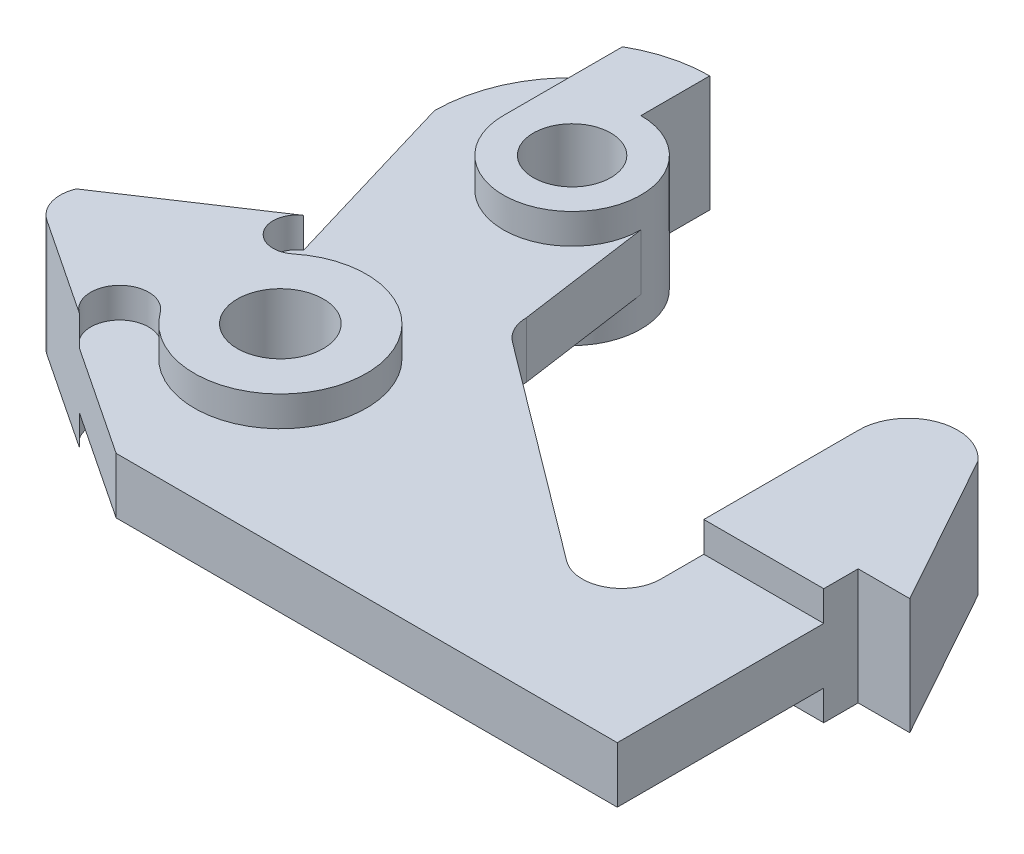
ISO-10303-21;
HEADER;
FILE_DESCRIPTION(('STEP AP214'),'2;1');
FILE_NAME('part.step','',(''),(''),'','','');
FILE_SCHEMA(('AUTOMOTIVE_DESIGN { 1 0 10303 214 1 1 1 1 }'));
ENDSEC;
DATA;
#1=APPLICATION_CONTEXT('core data for automotive mechanical design processes');
#2=APPLICATION_PROTOCOL_DEFINITION('international standard','automotive_design',2000,#1);
#3=PRODUCT_CONTEXT('',#1,'mechanical');
#4=PRODUCT('Part','Part','',(#3));
#5=PRODUCT_RELATED_PRODUCT_CATEGORY('part','',(#4));
#6=PRODUCT_DEFINITION_FORMATION('','',#4);
#7=PRODUCT_DEFINITION_CONTEXT('part definition',#1,'design');
#8=PRODUCT_DEFINITION('design','',#6,#7);
#9=PRODUCT_DEFINITION_SHAPE('','',#8);
#10=(LENGTH_UNIT() NAMED_UNIT(*) SI_UNIT(.MILLI.,.METRE.));
#11=(NAMED_UNIT(*) PLANE_ANGLE_UNIT() SI_UNIT($,.RADIAN.));
#12=(NAMED_UNIT(*) SI_UNIT($,.STERADIAN.) SOLID_ANGLE_UNIT());
#13=UNCERTAINTY_MEASURE_WITH_UNIT(LENGTH_MEASURE(1.E-05),#10,'distance_accuracy_value','');
#14=(GEOMETRIC_REPRESENTATION_CONTEXT(3) GLOBAL_UNCERTAINTY_ASSIGNED_CONTEXT((#13)) GLOBAL_UNIT_ASSIGNED_CONTEXT((#10,
#11,#12)) REPRESENTATION_CONTEXT('',''));
#15=CARTESIAN_POINT('',(0.,0.,0.));
#16=DIRECTION('',(0.,0.,1.));
#17=DIRECTION('',(1.,0.,0.));
#18=AXIS2_PLACEMENT_3D('',#15,#16,#17);
#19=CARTESIAN_POINT('',(0.,13.,0.));
#20=DIRECTION('',(0.,1.,0.));
#21=DIRECTION('',(0.,0.,1.));
#22=AXIS2_PLACEMENT_3D('',#19,#20,#21);
#23=PLANE('',#22);
#24=DIRECTION('',(0.,0.,-1.));
#25=VECTOR('',#24,1.);
#26=CARTESIAN_POINT('',(0.,13.,0.));
#27=LINE('',#26,#25);
#28=CARTESIAN_POINT('',(0.,13.,0.));
#29=VERTEX_POINT('',#28);
#30=CARTESIAN_POINT('',(0.,13.,-48.));
#31=VERTEX_POINT('',#30);
#32=EDGE_CURVE('E60',#29,#31,#27,.T.);
#33=ORIENTED_EDGE('',*,*,#32,.T.);
#34=DIRECTION('',(-1.,0.,0.));
#35=VECTOR('',#34,1.);
#36=CARTESIAN_POINT('',(0.,13.,-48.));
#37=LINE('',#36,#35);
#38=CARTESIAN_POINT('',(-27.8756729232547,13.,-48.));
#39=VERTEX_POINT('',#38);
#40=EDGE_CURVE('E63',#31,#39,#37,.T.);
#41=ORIENTED_EDGE('',*,*,#40,.T.);
#42=DIRECTION('',(0.,0.,1.));
#43=VECTOR('',#42,1.);
#44=CARTESIAN_POINT('',(-27.8756729232547,13.,0.));
#45=LINE('',#44,#43);
#46=CARTESIAN_POINT('',(-27.8756729232547,13.,-38.));
#47=VERTEX_POINT('',#46);
#48=EDGE_CURVE('E420',#39,#47,#45,.T.);
#49=ORIENTED_EDGE('',*,*,#48,.T.);
#50=CARTESIAN_POINT('',(-37.,13.,-38.));
#51=DIRECTION('',(0.,1.,0.));
#52=DIRECTION('',(0.,0.,1.));
#53=AXIS2_PLACEMENT_3D('',#50,#51,#52);
#54=CIRCLE('',#53,9.12432707674531);
#55=CARTESIAN_POINT('',(-42.4745962460472,13.,-30.7005383386037));
#56=VERTEX_POINT('',#55);
#57=EDGE_CURVE('E423',#56,#47,#54,.T.);
#58=ORIENTED_EDGE('',*,*,#57,.F.);
#59=DIRECTION('',(0.800000000000001,0.,0.599999999999999));
#60=VECTOR('',#59,1.);
#61=CARTESIAN_POINT('',(-0.554596246047137,13.,0.739461661396186));
#62=LINE('',#61,#60);
#63=CARTESIAN_POINT('',(-92.8745962460472,13.,-68.5005383386037));
#64=VERTEX_POINT('',#63);
#65=EDGE_CURVE('E424',#64,#56,#62,.T.);
#66=ORIENTED_EDGE('',*,*,#65,.F.);
#67=CARTESIAN_POINT('',(-88.,13.,-75.));
#68=DIRECTION('',(0.,1.,0.));
#69=DIRECTION('',(0.,0.,1.));
#70=AXIS2_PLACEMENT_3D('',#67,#68,#69);
#71=CIRCLE('',#70,8.12432707674541);
#72=CARTESIAN_POINT('',(-96.1243270767454,13.,-75.));
#73=VERTEX_POINT('',#72);
#74=EDGE_CURVE('E430',#73,#64,#71,.T.);
#75=ORIENTED_EDGE('',*,*,#74,.F.);
#76=DIRECTION('',(0.139765297021305,0.,0.990184660428824));
#77=VECTOR('',#76,1.);
#78=CARTESIAN_POINT('',(-83.8670929696268,13.,11.8379021890088));
#79=LINE('',#78,#77);
#80=CARTESIAN_POINT('',(-100.5,13.,-106.));
#81=VERTEX_POINT('',#80);
#82=EDGE_CURVE('E403',#81,#73,#79,.T.);
#83=ORIENTED_EDGE('',*,*,#82,.F.);
#84=CARTESIAN_POINT('',(-116.5,13.,-106.));
#85=DIRECTION('',(0.,1.,0.));
#86=DIRECTION('',(0.,0.,1.));
#87=AXIS2_PLACEMENT_3D('',#84,#85,#86);
#88=CIRCLE('',#87,16.);
#89=CARTESIAN_POINT('',(-132.5,13.,-106.));
#90=VERTEX_POINT('',#89);
#91=EDGE_CURVE('E338',#90,#81,#88,.T.);
#92=ORIENTED_EDGE('',*,*,#91,.F.);
#93=DIRECTION('',(0.,0.,-1.));
#94=VECTOR('',#93,1.);
#95=CARTESIAN_POINT('',(-132.5,13.,0.));
#96=LINE('',#95,#94);
#97=CARTESIAN_POINT('',(-132.5,13.,-133.712812921102));
#98=VERTEX_POINT('',#97);
#99=EDGE_CURVE('E341',#90,#98,#96,.T.);
#100=ORIENTED_EDGE('',*,*,#99,.T.);
#101=CARTESIAN_POINT('',(-116.5,13.,-106.));
#102=DIRECTION('',(0.,1.,0.));
#103=DIRECTION('',(0.,0.,1.));
#104=AXIS2_PLACEMENT_3D('',#101,#102,#103);
#105=CIRCLE('',#104,32.);
#106=CARTESIAN_POINT('',(-148.5,13.,-106.));
#107=VERTEX_POINT('',#106);
#108=EDGE_CURVE('E406',#98,#107,#105,.T.);
#109=ORIENTED_EDGE('',*,*,#108,.T.);
#110=DIRECTION('',(0.285281814189651,0.,0.958443679353493));
#111=VECTOR('',#110,1.);
#112=CARTESIAN_POINT('',(-107.431007069836,13.,31.9769572874406));
#113=LINE('',#112,#111);
#114=CARTESIAN_POINT('',(-135.615390406739,13.,-62.7123734799689));
#115=VERTEX_POINT('',#114);
#116=EDGE_CURVE('E413',#107,#115,#113,.T.);
#117=ORIENTED_EDGE('',*,*,#116,.T.);
#118=CARTESIAN_POINT('',(-132.537393975841,13.,-58.0787315938849));
#119=DIRECTION('',(0.,1.,0.));
#120=DIRECTION('',(0.,0.,1.));
#121=AXIS2_PLACEMENT_3D('',#118,#119,#120);
#122=CIRCLE('',#121,5.56279598377384);
#123=CARTESIAN_POINT('',(-129.047449023981,13.,-53.7468747876095));
#124=VERTEX_POINT('',#123);
#125=EDGE_CURVE('E402',#124,#115,#122,.F.);
#126=ORIENTED_EDGE('',*,*,#125,.F.);
#127=CARTESIAN_POINT('',(-116.5,13.,-38.172488026308));
#128=DIRECTION('',(0.,1.,0.));
#129=DIRECTION('',(0.,0.,1.));
#130=AXIS2_PLACEMENT_3D('',#127,#128,#129);
#131=CIRCLE('',#130,20.);
#132=CARTESIAN_POINT('',(-132.69631346136,13.,-26.4388001890858));
#133=VERTEX_POINT('',#132);
#134=EDGE_CURVE('E399',#133,#124,#131,.T.);
#135=ORIENTED_EDGE('',*,*,#134,.F.);
#136=CARTESIAN_POINT('',(-138.15745595221,13.,-22.4823849607005));
#137=DIRECTION('',(0.,1.,0.));
#138=DIRECTION('',(0.,0.,1.));
#139=AXIS2_PLACEMENT_3D('',#136,#137,#138);
#140=CIRCLE('',#139,6.74368584416329);
#141=CARTESIAN_POINT('',(-141.888860271185,13.,-16.8650973080069));
#142=VERTEX_POINT('',#141);
#143=EDGE_CURVE('E384',#142,#133,#140,.F.);
#144=ORIENTED_EDGE('',*,*,#143,.F.);
#145=DIRECTION('',(0.832969948853045,0.,0.553318230594073));
#146=VECTOR('',#145,1.);
#147=CARTESIAN_POINT('',(-35.6677639918536,13.,53.6945538846574));
#148=LINE('',#147,#146);
#149=CARTESIAN_POINT('',(-116.5,13.,0.));
#150=VERTEX_POINT('',#149);
#151=EDGE_CURVE('E414',#142,#150,#148,.T.);
#152=ORIENTED_EDGE('',*,*,#151,.T.);
#153=DIRECTION('',(1.,0.,0.));
#154=VECTOR('',#153,1.);
#155=CARTESIAN_POINT('',(0.,13.,0.));
#156=LINE('',#155,#154);
#157=EDGE_CURVE('E418',#150,#29,#156,.T.);
#158=ORIENTED_EDGE('',*,*,#157,.T.);
#159=EDGE_LOOP('',(#33,#41,#49,#58,#66,#75,#83,#92,#100,#109,#117,#126,#135,#144,#152,#158));
#160=FACE_BOUND('',#159,.T.);
#161=ADVANCED_FACE('F45',(#160),#23,.T.);
#162=CARTESIAN_POINT('',(0.,0.,0.));
#163=DIRECTION('',(0.,1.,0.));
#164=DIRECTION('',(0.,0.,1.));
#165=AXIS2_PLACEMENT_3D('',#162,#163,#164);
#166=PLANE('',#165);
#167=DIRECTION('',(-1.,0.,0.));
#168=VECTOR('',#167,1.);
#169=CARTESIAN_POINT('',(0.,0.,-48.));
#170=LINE('',#169,#168);
#171=CARTESIAN_POINT('',(0.,0.,-48.));
#172=VERTEX_POINT('',#171);
#173=CARTESIAN_POINT('',(-27.8756729232547,0.,-48.));
#174=VERTEX_POINT('',#173);
#175=EDGE_CURVE('E304',#172,#174,#170,.T.);
#176=ORIENTED_EDGE('',*,*,#175,.F.);
#177=DIRECTION('',(0.,0.,-1.));
#178=VECTOR('',#177,1.);
#179=CARTESIAN_POINT('',(0.,0.,0.));
#180=LINE('',#179,#178);
#181=CARTESIAN_POINT('',(0.,0.,0.));
#182=VERTEX_POINT('',#181);
#183=EDGE_CURVE('E445',#182,#172,#180,.T.);
#184=ORIENTED_EDGE('',*,*,#183,.F.);
#185=DIRECTION('',(1.,0.,0.));
#186=VECTOR('',#185,1.);
#187=CARTESIAN_POINT('',(0.,0.,0.));
#188=LINE('',#187,#186);
#189=CARTESIAN_POINT('',(-116.5,0.,0.));
#190=VERTEX_POINT('',#189);
#191=EDGE_CURVE('E439',#190,#182,#188,.T.);
#192=ORIENTED_EDGE('',*,*,#191,.F.);
#193=DIRECTION('',(0.832969948853045,0.,0.553318230594073));
#194=VECTOR('',#193,1.);
#195=CARTESIAN_POINT('',(-35.6677639918536,0.,53.6945538846574));
#196=LINE('',#195,#194);
#197=CARTESIAN_POINT('',(-141.888860271185,0.,-16.8650973080069));
#198=VERTEX_POINT('',#197);
#199=EDGE_CURVE('E437',#198,#190,#196,.T.);
#200=ORIENTED_EDGE('',*,*,#199,.F.);
#201=CARTESIAN_POINT('',(-138.15745595221,0.,-22.4823849607005));
#202=DIRECTION('',(0.,1.,0.));
#203=DIRECTION('',(0.,0.,1.));
#204=AXIS2_PLACEMENT_3D('',#201,#202,#203);
#205=CIRCLE('',#204,6.74368584416329);
#206=CARTESIAN_POINT('',(-132.69631346136,0.,-26.4388001890858));
#207=VERTEX_POINT('',#206);
#208=EDGE_CURVE('E495',#198,#207,#205,.F.);
#209=ORIENTED_EDGE('',*,*,#208,.T.);
#210=CARTESIAN_POINT('',(-116.5,0.,-38.172488026308));
#211=DIRECTION('',(0.,1.,0.));
#212=DIRECTION('',(0.,0.,1.));
#213=AXIS2_PLACEMENT_3D('',#210,#211,#212);
#214=CIRCLE('',#213,20.);
#215=CARTESIAN_POINT('',(-129.047449023981,0.,-53.7468747876095));
#216=VERTEX_POINT('',#215);
#217=EDGE_CURVE('E493',#207,#216,#214,.T.);
#218=ORIENTED_EDGE('',*,*,#217,.T.);
#219=CARTESIAN_POINT('',(-132.537393975841,0.,-58.0787315938849));
#220=DIRECTION('',(0.,1.,0.));
#221=DIRECTION('',(0.,0.,1.));
#222=AXIS2_PLACEMENT_3D('',#219,#220,#221);
#223=CIRCLE('',#222,5.56279598377384);
#224=CARTESIAN_POINT('',(-135.615390406739,0.,-62.7123734799689));
#225=VERTEX_POINT('',#224);
#226=EDGE_CURVE('E497',#216,#225,#223,.F.);
#227=ORIENTED_EDGE('',*,*,#226,.T.);
#228=DIRECTION('',(0.285281814189651,0.,0.958443679353493));
#229=VECTOR('',#228,1.);
#230=CARTESIAN_POINT('',(-107.431007069836,0.,31.9769572874406));
#231=LINE('',#230,#229);
#232=CARTESIAN_POINT('',(-148.5,0.,-106.));
#233=VERTEX_POINT('',#232);
#234=EDGE_CURVE('E434',#233,#225,#231,.T.);
#235=ORIENTED_EDGE('',*,*,#234,.F.);
#236=CARTESIAN_POINT('',(-116.5,0.,-106.));
#237=DIRECTION('',(0.,1.,0.));
#238=DIRECTION('',(0.,0.,1.));
#239=AXIS2_PLACEMENT_3D('',#236,#237,#238);
#240=CIRCLE('',#239,32.);
#241=CARTESIAN_POINT('',(-132.5,0.,-133.712812921102));
#242=VERTEX_POINT('',#241);
#243=EDGE_CURVE('E433',#242,#233,#240,.T.);
#244=ORIENTED_EDGE('',*,*,#243,.F.);
#245=DIRECTION('',(0.,0.,-1.));
#246=VECTOR('',#245,1.);
#247=CARTESIAN_POINT('',(-132.5,0.,0.));
#248=LINE('',#247,#246);
#249=CARTESIAN_POINT('',(-132.5,0.,-106.));
#250=VERTEX_POINT('',#249);
#251=EDGE_CURVE('E12',#250,#242,#248,.T.);
#252=ORIENTED_EDGE('',*,*,#251,.F.);
#253=CARTESIAN_POINT('',(-116.5,0.,-106.));
#254=DIRECTION('',(0.,1.,0.));
#255=DIRECTION('',(0.,0.,1.));
#256=AXIS2_PLACEMENT_3D('',#253,#254,#255);
#257=CIRCLE('',#256,16.);
#258=CARTESIAN_POINT('',(-100.5,0.,-106.));
#259=VERTEX_POINT('',#258);
#260=EDGE_CURVE('E49',#250,#259,#257,.T.);
#261=ORIENTED_EDGE('',*,*,#260,.T.);
#262=DIRECTION('',(0.139765297021305,0.,0.990184660428824));
#263=VECTOR('',#262,1.);
#264=CARTESIAN_POINT('',(-83.8670929696268,0.,11.8379021890088));
#265=LINE('',#264,#263);
#266=CARTESIAN_POINT('',(-96.1243270767454,0.,-75.));
#267=VERTEX_POINT('',#266);
#268=EDGE_CURVE('E404',#259,#267,#265,.T.);
#269=ORIENTED_EDGE('',*,*,#268,.T.);
#270=CARTESIAN_POINT('',(-88.,0.,-75.));
#271=DIRECTION('',(0.,1.,0.));
#272=DIRECTION('',(0.,0.,1.));
#273=AXIS2_PLACEMENT_3D('',#270,#271,#272);
#274=CIRCLE('',#273,8.12432707674541);
#275=CARTESIAN_POINT('',(-92.8745962460472,0.,-68.5005383386037));
#276=VERTEX_POINT('',#275);
#277=EDGE_CURVE('E409',#267,#276,#274,.T.);
#278=ORIENTED_EDGE('',*,*,#277,.T.);
#279=DIRECTION('',(0.800000000000001,0.,0.599999999999999));
#280=VECTOR('',#279,1.);
#281=CARTESIAN_POINT('',(-0.554596246047137,0.,0.739461661396186));
#282=LINE('',#281,#280);
#283=CARTESIAN_POINT('',(-42.4745962460472,0.,-30.7005383386037));
#284=VERTEX_POINT('',#283);
#285=EDGE_CURVE('E447',#276,#284,#282,.T.);
#286=ORIENTED_EDGE('',*,*,#285,.T.);
#287=CARTESIAN_POINT('',(-37.,0.,-38.));
#288=DIRECTION('',(0.,1.,0.));
#289=DIRECTION('',(0.,0.,1.));
#290=AXIS2_PLACEMENT_3D('',#287,#288,#289);
#291=CIRCLE('',#290,9.12432707674531);
#292=CARTESIAN_POINT('',(-27.8756729232547,0.,-38.));
#293=VERTEX_POINT('',#292);
#294=EDGE_CURVE('E450',#284,#293,#291,.T.);
#295=ORIENTED_EDGE('',*,*,#294,.T.);
#296=DIRECTION('',(0.,0.,1.));
#297=VECTOR('',#296,1.);
#298=CARTESIAN_POINT('',(-27.8756729232547,0.,0.));
#299=LINE('',#298,#297);
#300=EDGE_CURVE('E443',#174,#293,#299,.T.);
#301=ORIENTED_EDGE('',*,*,#300,.F.);
#302=EDGE_LOOP('',(#176,#184,#192,#200,#209,#218,#227,#235,#244,#252,#261,#269,#278,#286,#295,#301));
#303=FACE_BOUND('',#302,.T.);
#304=ADVANCED_FACE('F503',(#303),#166,.F.);
#305=CARTESIAN_POINT('',(-83.8670929696268,13.,11.8379021890088));
#306=DIRECTION('',(0.990184660428824,0.,-0.139765297021305));
#307=DIRECTION('',(-0.139765297021305,0.,-0.990184660428824));
#308=AXIS2_PLACEMENT_3D('',#305,#306,#307);
#309=PLANE('',#308);
#310=ORIENTED_EDGE('',*,*,#268,.F.);
#311=DIRECTION('',(0.,-1.,0.));
#312=VECTOR('',#311,1.);
#313=CARTESIAN_POINT('',(-100.5,13.,-106.));
#314=LINE('',#313,#312);
#315=EDGE_CURVE('E487',#81,#259,#314,.T.);
#316=ORIENTED_EDGE('',*,*,#315,.F.);
#317=ORIENTED_EDGE('',*,*,#82,.T.);
#318=DIRECTION('',(0.,-1.,0.));
#319=VECTOR('',#318,1.);
#320=CARTESIAN_POINT('',(-96.1243270767454,13.,-75.));
#321=LINE('',#320,#319);
#322=EDGE_CURVE('E429',#73,#267,#321,.T.);
#323=ORIENTED_EDGE('',*,*,#322,.T.);
#324=EDGE_LOOP('',(#310,#316,#317,#323));
#325=FACE_BOUND('',#324,.T.);
#326=ADVANCED_FACE('F42',(#325),#309,.T.);
#327=CARTESIAN_POINT('',(-116.5,13.,-106.));
#328=DIRECTION('',(0.,-1.,0.));
#329=DIRECTION('',(0.,0.,-1.));
#330=AXIS2_PLACEMENT_3D('',#327,#328,#329);
#331=CYLINDRICAL_SURFACE('',#330,16.);
#332=ORIENTED_EDGE('',*,*,#315,.T.);
#333=ORIENTED_EDGE('',*,*,#260,.F.);
#334=DIRECTION('',(0.,1.,0.));
#335=VECTOR('',#334,1.);
#336=CARTESIAN_POINT('',(-132.5,-7.,-106.));
#337=LINE('',#336,#335);
#338=CARTESIAN_POINT('',(-132.5,-7.,-106.));
#339=VERTEX_POINT('',#338);
#340=EDGE_CURVE('E336',#339,#250,#337,.T.);
#341=ORIENTED_EDGE('',*,*,#340,.F.);
#342=CARTESIAN_POINT('',(-116.5,-7.,-106.));
#343=DIRECTION('',(0.,1.,0.));
#344=DIRECTION('',(0.,0.,1.));
#345=AXIS2_PLACEMENT_3D('',#342,#343,#344);
#346=CIRCLE('',#345,16.);
#347=CARTESIAN_POINT('',(-116.5,-7.,-122.));
#348=VERTEX_POINT('',#347);
#349=EDGE_CURVE('E323',#339,#348,#346,.T.);
#350=ORIENTED_EDGE('',*,*,#349,.T.);
#351=DIRECTION('',(0.,-1.,0.));
#352=VECTOR('',#351,1.);
#353=CARTESIAN_POINT('',(-116.5,13.,-122.));
#354=LINE('',#353,#352);
#355=CARTESIAN_POINT('',(-116.5,20.,-122.));
#356=VERTEX_POINT('',#355);
#357=EDGE_CURVE('E490',#356,#348,#354,.T.);
#358=ORIENTED_EDGE('',*,*,#357,.F.);
#359=CARTESIAN_POINT('',(-116.5,20.,-106.));
#360=DIRECTION('',(0.,1.,0.));
#361=DIRECTION('',(0.,0.,1.));
#362=AXIS2_PLACEMENT_3D('',#359,#360,#361);
#363=CIRCLE('',#362,16.);
#364=CARTESIAN_POINT('',(-132.5,20.,-106.));
#365=VERTEX_POINT('',#364);
#366=EDGE_CURVE('E315',#365,#356,#363,.T.);
#367=ORIENTED_EDGE('',*,*,#366,.F.);
#368=EDGE_CURVE('E335',#90,#365,#337,.T.);
#369=ORIENTED_EDGE('',*,*,#368,.F.);
#370=ORIENTED_EDGE('',*,*,#91,.T.);
#371=EDGE_LOOP('',(#332,#333,#341,#350,#358,#367,#369,#370));
#372=FACE_BOUND('',#371,.T.);
#373=ADVANCED_FACE('F510',(#372),#331,.T.);
#374=CARTESIAN_POINT('',(-116.499999999999,13.,8.08381139805186E-13));
#375=DIRECTION('',(-1.,0.,0.));
#376=DIRECTION('',(0.,0.,1.));
#377=AXIS2_PLACEMENT_3D('',#374,#375,#376);
#378=PLANE('',#377);
#379=ORIENTED_EDGE('',*,*,#357,.T.);
#380=DIRECTION('',(0.,0.,-1.));
#381=VECTOR('',#380,1.);
#382=CARTESIAN_POINT('',(-116.499999999999,-7.,8.08381139805186E-13));
#383=LINE('',#382,#381);
#384=CARTESIAN_POINT('',(-116.5,-7.,-138.));
#385=VERTEX_POINT('',#384);
#386=EDGE_CURVE('E326',#348,#385,#383,.T.);
#387=ORIENTED_EDGE('',*,*,#386,.T.);
#388=DIRECTION('',(0.,-1.,0.));
#389=VECTOR('',#388,1.);
#390=CARTESIAN_POINT('',(-116.5,13.,-138.));
#391=LINE('',#390,#389);
#392=CARTESIAN_POINT('',(-116.5,20.,-138.));
#393=VERTEX_POINT('',#392);
#394=EDGE_CURVE('E484',#393,#385,#391,.T.);
#395=ORIENTED_EDGE('',*,*,#394,.F.);
#396=DIRECTION('',(0.,0.,-1.));
#397=VECTOR('',#396,1.);
#398=CARTESIAN_POINT('',(-116.499999999999,20.,8.08381139805186E-13));
#399=LINE('',#398,#397);
#400=EDGE_CURVE('E312',#356,#393,#399,.T.);
#401=ORIENTED_EDGE('',*,*,#400,.F.);
#402=EDGE_LOOP('',(#379,#387,#395,#401));
#403=FACE_BOUND('',#402,.T.);
#404=ADVANCED_FACE('F635',(#403),#378,.F.);
#405=CARTESIAN_POINT('',(-116.5,13.,-106.));
#406=DIRECTION('',(0.,-1.,0.));
#407=DIRECTION('',(0.,0.,-1.));
#408=AXIS2_PLACEMENT_3D('',#405,#406,#407);
#409=CYLINDRICAL_SURFACE('',#408,32.);
#410=ORIENTED_EDGE('',*,*,#394,.T.);
#411=CARTESIAN_POINT('',(-116.5,-7.,-106.));
#412=DIRECTION('',(0.,1.,0.));
#413=DIRECTION('',(0.,0.,1.));
#414=AXIS2_PLACEMENT_3D('',#411,#412,#413);
#415=CIRCLE('',#414,32.);
#416=CARTESIAN_POINT('',(-132.5,-7.,-133.712812921102));
#417=VERTEX_POINT('',#416);
#418=EDGE_CURVE('E328',#385,#417,#415,.T.);
#419=ORIENTED_EDGE('',*,*,#418,.T.);
#420=DIRECTION('',(0.,1.,0.));
#421=VECTOR('',#420,1.);
#422=CARTESIAN_POINT('',(-132.5,-7.,-133.712812921102));
#423=LINE('',#422,#421);
#424=EDGE_CURVE('E334',#417,#242,#423,.T.);
#425=ORIENTED_EDGE('',*,*,#424,.T.);
#426=ORIENTED_EDGE('',*,*,#243,.T.);
#427=DIRECTION('',(0.,-1.,0.));
#428=VECTOR('',#427,1.);
#429=CARTESIAN_POINT('',(-148.5,13.,-106.));
#430=LINE('',#429,#428);
#431=EDGE_CURVE('E485',#107,#233,#430,.T.);
#432=ORIENTED_EDGE('',*,*,#431,.F.);
#433=ORIENTED_EDGE('',*,*,#108,.F.);
#434=CARTESIAN_POINT('',(-132.5,20.,-133.712812921102));
#435=VERTEX_POINT('',#434);
#436=EDGE_CURVE('E340',#98,#435,#423,.T.);
#437=ORIENTED_EDGE('',*,*,#436,.T.);
#438=CARTESIAN_POINT('',(-116.5,20.,-106.));
#439=DIRECTION('',(0.,1.,0.));
#440=DIRECTION('',(0.,0.,1.));
#441=AXIS2_PLACEMENT_3D('',#438,#439,#440);
#442=CIRCLE('',#441,32.);
#443=EDGE_CURVE('E318',#393,#435,#442,.T.);
#444=ORIENTED_EDGE('',*,*,#443,.F.);
#445=EDGE_LOOP('',(#410,#419,#425,#426,#432,#433,#437,#444));
#446=FACE_BOUND('',#445,.T.);
#447=ADVANCED_FACE('F629',(#446),#409,.T.);
#448=CARTESIAN_POINT('',(-107.431007069836,13.,31.9769572874406));
#449=DIRECTION('',(0.958443679353493,0.,-0.285281814189651));
#450=DIRECTION('',(-0.285281814189651,0.,-0.958443679353493));
#451=AXIS2_PLACEMENT_3D('',#448,#449,#450);
#452=PLANE('',#451);
#453=DIRECTION('',(0.,-1.,0.));
#454=VECTOR('',#453,1.);
#455=CARTESIAN_POINT('',(-135.615390406739,13.,-62.7123734799689));
#456=LINE('',#455,#454);
#457=EDGE_CURVE('E477',#115,#225,#456,.T.);
#458=ORIENTED_EDGE('',*,*,#457,.F.);
#459=ORIENTED_EDGE('',*,*,#116,.F.);
#460=ORIENTED_EDGE('',*,*,#431,.T.);
#461=ORIENTED_EDGE('',*,*,#234,.T.);
#462=EDGE_LOOP('',(#458,#459,#460,#461));
#463=FACE_BOUND('',#462,.T.);
#464=ADVANCED_FACE('F569',(#463),#452,.F.);
#465=CARTESIAN_POINT('',(-70.4241258003915,13.,-106.017075206415));
#466=DIRECTION('',(-0.553318230594074,0.,-0.832969948853044));
#467=DIRECTION('',(-0.832969948853044,0.,0.553318230594074));
#468=AXIS2_PLACEMENT_3D('',#465,#466,#467);
#469=PLANE('',#468);
#470=ORIENTED_EDGE('',*,*,#457,.T.);
#471=DIRECTION('',(0.,1.,0.));
#472=VECTOR('',#471,1.);
#473=CARTESIAN_POINT('',(-135.615390406739,-7.,-62.7123734799689));
#474=LINE('',#473,#472);
#475=CARTESIAN_POINT('',(-135.615390406739,-7.,-62.7123734799689));
#476=VERTEX_POINT('',#475);
#477=EDGE_CURVE('E392',#476,#225,#474,.T.);
#478=ORIENTED_EDGE('',*,*,#477,.F.);
#479=DIRECTION('',(-0.832969948853044,0.,0.553318230594074));
#480=VECTOR('',#479,1.);
#481=CARTESIAN_POINT('',(-135.615390406739,-7.,-62.7123734799689));
#482=LINE('',#481,#480);
#483=CARTESIAN_POINT('',(-167.365927817775,-7.,-41.6213951020864));
#484=VERTEX_POINT('',#483);
#485=EDGE_CURVE('E368',#476,#484,#482,.T.);
#486=ORIENTED_EDGE('',*,*,#485,.T.);
#487=DIRECTION('',(0.,-1.,0.));
#488=VECTOR('',#487,1.);
#489=CARTESIAN_POINT('',(-167.365927817775,13.,-41.6213951020864));
#490=LINE('',#489,#488);
#491=CARTESIAN_POINT('',(-167.365927817775,20.,-41.6213951020864));
#492=VERTEX_POINT('',#491);
#493=EDGE_CURVE('E476',#492,#484,#490,.T.);
#494=ORIENTED_EDGE('',*,*,#493,.F.);
#495=DIRECTION('',(-0.832969948853044,0.,0.553318230594074));
#496=VECTOR('',#495,1.);
#497=CARTESIAN_POINT('',(-135.615390406739,20.,-62.7123734799689));
#498=LINE('',#497,#496);
#499=CARTESIAN_POINT('',(-135.615390406739,20.,-62.7123734799689));
#500=VERTEX_POINT('',#499);
#501=EDGE_CURVE('E346',#500,#492,#498,.T.);
#502=ORIENTED_EDGE('',*,*,#501,.F.);
#503=EDGE_CURVE('E381',#115,#500,#474,.T.);
#504=ORIENTED_EDGE('',*,*,#503,.F.);
#505=EDGE_LOOP('',(#470,#478,#486,#494,#502,#504));
#506=FACE_BOUND('',#505,.T.);
#507=ADVANCED_FACE('F558',(#506),#469,.T.);
#508=CARTESIAN_POINT('',(-160.,13.,-38.5));
#509=DIRECTION('',(0.,-1.,0.));
#510=DIRECTION('',(0.,0.,-1.));
#511=AXIS2_PLACEMENT_3D('',#508,#509,#510);
#512=CYLINDRICAL_SURFACE('',#511,8.00000000000002);
#513=ORIENTED_EDGE('',*,*,#493,.T.);
#514=CARTESIAN_POINT('',(-160.,-7.,-38.5));
#515=DIRECTION('',(0.,1.,0.));
#516=DIRECTION('',(0.,0.,1.));
#517=AXIS2_PLACEMENT_3D('',#514,#515,#516);
#518=CIRCLE('',#517,8.);
#519=CARTESIAN_POINT('',(-164.426545844753,-7.,-31.8362404091756));
#520=VERTEX_POINT('',#519);
#521=EDGE_CURVE('E369',#484,#520,#518,.T.);
#522=ORIENTED_EDGE('',*,*,#521,.T.);
#523=DIRECTION('',(0.,-1.,0.));
#524=VECTOR('',#523,1.);
#525=CARTESIAN_POINT('',(-164.426545844753,13.,-31.8362404091756));
#526=LINE('',#525,#524);
#527=CARTESIAN_POINT('',(-164.426545844753,20.,-31.8362404091756));
#528=VERTEX_POINT('',#527);
#529=EDGE_CURVE('E478',#528,#520,#526,.T.);
#530=ORIENTED_EDGE('',*,*,#529,.F.);
#531=CARTESIAN_POINT('',(-160.,20.,-38.5));
#532=DIRECTION('',(0.,1.,0.));
#533=DIRECTION('',(0.,0.,1.));
#534=AXIS2_PLACEMENT_3D('',#531,#532,#533);
#535=CIRCLE('',#534,8.);
#536=EDGE_CURVE('E353',#492,#528,#535,.T.);
#537=ORIENTED_EDGE('',*,*,#536,.F.);
#538=EDGE_LOOP('',(#513,#522,#530,#537));
#539=FACE_BOUND('',#538,.T.);
#540=ADVANCED_FACE('F555',(#539),#512,.T.);
#541=CARTESIAN_POINT('',(-35.6677639918536,13.,53.6945538846574));
#542=DIRECTION('',(0.553318230594073,0.,-0.832969948853045));
#543=DIRECTION('',(-0.832969948853045,0.,-0.553318230594073));
#544=AXIS2_PLACEMENT_3D('',#541,#542,#543);
#545=PLANE('',#544);
#546=ORIENTED_EDGE('',*,*,#151,.F.);
#547=DIRECTION('',(0.,1.,0.));
#548=VECTOR('',#547,1.);
#549=CARTESIAN_POINT('',(-141.888860271185,-7.,-16.8650973080069));
#550=LINE('',#549,#548);
#551=CARTESIAN_POINT('',(-141.888860271185,20.,-16.8650973080069));
#552=VERTEX_POINT('',#551);
#553=EDGE_CURVE('E394',#142,#552,#550,.T.);
#554=ORIENTED_EDGE('',*,*,#553,.T.);
#555=DIRECTION('',(0.832969948853045,0.,0.553318230594073));
#556=VECTOR('',#555,1.);
#557=CARTESIAN_POINT('',(-141.888860271185,20.,-16.8650973080069));
#558=LINE('',#557,#556);
#559=EDGE_CURVE('E354',#528,#552,#558,.T.);
#560=ORIENTED_EDGE('',*,*,#559,.F.);
#561=ORIENTED_EDGE('',*,*,#529,.T.);
#562=DIRECTION('',(0.832969948853045,0.,0.553318230594073));
#563=VECTOR('',#562,1.);
#564=CARTESIAN_POINT('',(-141.888860271185,-7.,-16.8650973080069));
#565=LINE('',#564,#563);
#566=CARTESIAN_POINT('',(-141.888860271185,-7.,-16.8650973080069));
#567=VERTEX_POINT('',#566);
#568=EDGE_CURVE('E375',#520,#567,#565,.T.);
#569=ORIENTED_EDGE('',*,*,#568,.T.);
#570=EDGE_CURVE('E393',#567,#198,#550,.T.);
#571=ORIENTED_EDGE('',*,*,#570,.T.);
#572=ORIENTED_EDGE('',*,*,#199,.T.);
#573=DIRECTION('',(0.,-1.,0.));
#574=VECTOR('',#573,1.);
#575=CARTESIAN_POINT('',(-116.5,13.,0.));
#576=LINE('',#575,#574);
#577=EDGE_CURVE('E471',#150,#190,#576,.T.);
#578=ORIENTED_EDGE('',*,*,#577,.F.);
#579=EDGE_LOOP('',(#546,#554,#560,#561,#569,#571,#572,#578));
#580=FACE_BOUND('',#579,.T.);
#581=ADVANCED_FACE('F545',(#580),#545,.F.);
#582=CARTESIAN_POINT('',(0.,13.,0.));
#583=DIRECTION('',(0.,0.,-1.));
#584=DIRECTION('',(-1.,0.,0.));
#585=AXIS2_PLACEMENT_3D('',#582,#583,#584);
#586=PLANE('',#585);
#587=ORIENTED_EDGE('',*,*,#191,.T.);
#588=DIRECTION('',(0.,-1.,0.));
#589=VECTOR('',#588,1.);
#590=CARTESIAN_POINT('',(0.,13.,0.));
#591=LINE('',#590,#589);
#592=EDGE_CURVE('E467',#29,#182,#591,.T.);
#593=ORIENTED_EDGE('',*,*,#592,.F.);
#594=ORIENTED_EDGE('',*,*,#157,.F.);
#595=ORIENTED_EDGE('',*,*,#577,.T.);
#596=EDGE_LOOP('',(#587,#593,#594,#595));
#597=FACE_BOUND('',#596,.T.);
#598=ADVANCED_FACE('F531',(#597),#586,.F.);
#599=CARTESIAN_POINT('',(0.,13.,0.));
#600=DIRECTION('',(-1.,0.,0.));
#601=DIRECTION('',(0.,0.,1.));
#602=AXIS2_PLACEMENT_3D('',#599,#600,#601);
#603=PLANE('',#602);
#604=DIRECTION('',(0.,-1.,0.));
#605=VECTOR('',#604,1.);
#606=CARTESIAN_POINT('',(0.,13.,-56.));
#607=LINE('',#606,#605);
#608=CARTESIAN_POINT('',(0.,20.,-56.));
#609=VERTEX_POINT('',#608);
#610=CARTESIAN_POINT('',(0.,-7.,-56.));
#611=VERTEX_POINT('',#610);
#612=EDGE_CURVE('E265',#609,#611,#607,.T.);
#613=ORIENTED_EDGE('',*,*,#612,.F.);
#614=DIRECTION('',(0.,0.,-1.));
#615=VECTOR('',#614,1.);
#616=CARTESIAN_POINT('',(0.,20.,0.));
#617=LINE('',#616,#615);
#618=CARTESIAN_POINT('',(0.,20.,-48.));
#619=VERTEX_POINT('',#618);
#620=EDGE_CURVE('E259',#619,#609,#617,.T.);
#621=ORIENTED_EDGE('',*,*,#620,.F.);
#622=DIRECTION('',(0.,1.,0.));
#623=VECTOR('',#622,1.);
#624=CARTESIAN_POINT('',(0.,-7.,-48.));
#625=LINE('',#624,#623);
#626=EDGE_CURVE('E246',#31,#619,#625,.T.);
#627=ORIENTED_EDGE('',*,*,#626,.F.);
#628=ORIENTED_EDGE('',*,*,#32,.F.);
#629=ORIENTED_EDGE('',*,*,#592,.T.);
#630=ORIENTED_EDGE('',*,*,#183,.T.);
#631=CARTESIAN_POINT('',(0.,-7.,-48.));
#632=VERTEX_POINT('',#631);
#633=EDGE_CURVE('E254',#632,#172,#625,.T.);
#634=ORIENTED_EDGE('',*,*,#633,.F.);
#635=DIRECTION('',(0.,0.,-1.));
#636=VECTOR('',#635,1.);
#637=CARTESIAN_POINT('',(0.,-7.,0.));
#638=LINE('',#637,#636);
#639=EDGE_CURVE('E289',#632,#611,#638,.T.);
#640=ORIENTED_EDGE('',*,*,#639,.T.);
#641=EDGE_LOOP('',(#613,#621,#627,#628,#629,#630,#634,#640));
#642=FACE_BOUND('',#641,.T.);
#643=ADVANCED_FACE('F257',(#642),#603,.F.);
#644=CARTESIAN_POINT('',(0.,13.,-56.));
#645=DIRECTION('',(0.,0.,-1.));
#646=DIRECTION('',(-1.,0.,0.));
#647=AXIS2_PLACEMENT_3D('',#644,#645,#646);
#648=PLANE('',#647);
#649=ORIENTED_EDGE('',*,*,#612,.T.);
#650=DIRECTION('',(1.,0.,0.));
#651=VECTOR('',#650,1.);
#652=CARTESIAN_POINT('',(0.,-7.,-56.));
#653=LINE('',#652,#651);
#654=CARTESIAN_POINT('',(12.,-7.,-56.));
#655=VERTEX_POINT('',#654);
#656=EDGE_CURVE('E292',#611,#655,#653,.T.);
#657=ORIENTED_EDGE('',*,*,#656,.T.);
#658=DIRECTION('',(0.,-1.,0.));
#659=VECTOR('',#658,1.);
#660=CARTESIAN_POINT('',(12.,13.,-56.));
#661=LINE('',#660,#659);
#662=CARTESIAN_POINT('',(12.,20.,-56.));
#663=VERTEX_POINT('',#662);
#664=EDGE_CURVE('E470',#663,#655,#661,.T.);
#665=ORIENTED_EDGE('',*,*,#664,.F.);
#666=DIRECTION('',(1.,0.,0.));
#667=VECTOR('',#666,1.);
#668=CARTESIAN_POINT('',(0.,20.,-56.));
#669=LINE('',#668,#667);
#670=EDGE_CURVE('E266',#609,#663,#669,.T.);
#671=ORIENTED_EDGE('',*,*,#670,.F.);
#672=EDGE_LOOP('',(#649,#657,#665,#671));
#673=FACE_BOUND('',#672,.T.);
#674=ADVANCED_FACE('F615',(#673),#648,.F.);
#675=CARTESIAN_POINT('',(32.9314806035054,13.,-18.2688462912658));
#676=DIRECTION('',(-0.874454947822757,0.,0.485106734882437));
#677=DIRECTION('',(0.485106734882437,0.,0.874454947822757));
#678=AXIS2_PLACEMENT_3D('',#675,#676,#677);
#679=PLANE('',#678);
#680=ORIENTED_EDGE('',*,*,#664,.T.);
#681=DIRECTION('',(-0.485106734882437,0.,-0.874454947822757));
#682=VECTOR('',#681,1.);
#683=CARTESIAN_POINT('',(32.9314806035054,-7.,-18.2688462912658));
#684=LINE('',#683,#682);
#685=CARTESIAN_POINT('',(-7.7565108604844,-7.,-91.6131495017306));
#686=VERTEX_POINT('',#685);
#687=EDGE_CURVE('E294',#655,#686,#684,.T.);
#688=ORIENTED_EDGE('',*,*,#687,.T.);
#689=DIRECTION('',(0.,-1.,0.));
#690=VECTOR('',#689,1.);
#691=CARTESIAN_POINT('',(-7.7565108604844,13.,-91.6131495017306));
#692=LINE('',#691,#690);
#693=CARTESIAN_POINT('',(-7.7565108604844,20.,-91.6131495017306));
#694=VERTEX_POINT('',#693);
#695=EDGE_CURVE('E462',#694,#686,#692,.T.);
#696=ORIENTED_EDGE('',*,*,#695,.F.);
#697=DIRECTION('',(-0.485106734882437,0.,-0.874454947822757));
#698=VECTOR('',#697,1.);
#699=CARTESIAN_POINT('',(32.9314806035054,20.,-18.2688462912658));
#700=LINE('',#699,#698);
#701=EDGE_CURVE('E283',#663,#694,#700,.T.);
#702=ORIENTED_EDGE('',*,*,#701,.F.);
#703=EDGE_LOOP('',(#680,#688,#696,#702));
#704=FACE_BOUND('',#703,.T.);
#705=ADVANCED_FACE('F609',(#704),#679,.F.);
#706=CARTESIAN_POINT('',(-16.3756729232547,13.,-84.));
#707=DIRECTION('',(0.,-1.,0.));
#708=DIRECTION('',(0.,0.,-1.));
#709=AXIS2_PLACEMENT_3D('',#706,#707,#708);
#710=CYLINDRICAL_SURFACE('',#709,11.5);
#711=ORIENTED_EDGE('',*,*,#695,.T.);
#712=CARTESIAN_POINT('',(-16.3756729232547,-7.,-84.));
#713=DIRECTION('',(0.,1.,0.));
#714=DIRECTION('',(0.,0.,1.));
#715=AXIS2_PLACEMENT_3D('',#712,#713,#714);
#716=CIRCLE('',#715,11.5);
#717=CARTESIAN_POINT('',(-27.8756729232547,-7.,-84.));
#718=VERTEX_POINT('',#717);
#719=EDGE_CURVE('E300',#686,#718,#716,.T.);
#720=ORIENTED_EDGE('',*,*,#719,.T.);
#721=DIRECTION('',(0.,-1.,0.));
#722=VECTOR('',#721,1.);
#723=CARTESIAN_POINT('',(-27.8756729232547,13.,-84.));
#724=LINE('',#723,#722);
#725=CARTESIAN_POINT('',(-27.8756729232547,20.,-84.));
#726=VERTEX_POINT('',#725);
#727=EDGE_CURVE('E461',#726,#718,#724,.T.);
#728=ORIENTED_EDGE('',*,*,#727,.F.);
#729=CARTESIAN_POINT('',(-16.3756729232547,20.,-84.));
#730=DIRECTION('',(0.,1.,0.));
#731=DIRECTION('',(0.,0.,1.));
#732=AXIS2_PLACEMENT_3D('',#729,#730,#731);
#733=CIRCLE('',#732,11.5);
#734=EDGE_CURVE('E284',#694,#726,#733,.T.);
#735=ORIENTED_EDGE('',*,*,#734,.F.);
#736=EDGE_LOOP('',(#711,#720,#728,#735));
#737=FACE_BOUND('',#736,.T.);
#738=ADVANCED_FACE('F604',(#737),#710,.T.);
#739=CARTESIAN_POINT('',(-27.8756729232547,13.,0.));
#740=DIRECTION('',(1.,0.,0.));
#741=DIRECTION('',(0.,0.,-1.));
#742=AXIS2_PLACEMENT_3D('',#739,#740,#741);
#743=PLANE('',#742);
#744=ORIENTED_EDGE('',*,*,#727,.T.);
#745=DIRECTION('',(0.,0.,1.));
#746=VECTOR('',#745,1.);
#747=CARTESIAN_POINT('',(-27.8756729232547,-7.,0.));
#748=LINE('',#747,#746);
#749=CARTESIAN_POINT('',(-27.8756729232547,-7.,-48.));
#750=VERTEX_POINT('',#749);
#751=EDGE_CURVE('E258',#718,#750,#748,.T.);
#752=ORIENTED_EDGE('',*,*,#751,.T.);
#753=DIRECTION('',(0.,1.,0.));
#754=VECTOR('',#753,1.);
#755=CARTESIAN_POINT('',(-27.8756729232547,-7.,-48.));
#756=LINE('',#755,#754);
#757=EDGE_CURVE('E305',#750,#174,#756,.T.);
#758=ORIENTED_EDGE('',*,*,#757,.T.);
#759=ORIENTED_EDGE('',*,*,#300,.T.);
#760=DIRECTION('',(0.,-1.,0.));
#761=VECTOR('',#760,1.);
#762=CARTESIAN_POINT('',(-27.8756729232547,13.,-38.));
#763=LINE('',#762,#761);
#764=EDGE_CURVE('E458',#47,#293,#763,.T.);
#765=ORIENTED_EDGE('',*,*,#764,.F.);
#766=ORIENTED_EDGE('',*,*,#48,.F.);
#767=CARTESIAN_POINT('',(-27.8756729232547,20.,-48.));
#768=VERTEX_POINT('',#767);
#769=EDGE_CURVE('E302',#39,#768,#756,.T.);
#770=ORIENTED_EDGE('',*,*,#769,.T.);
#771=DIRECTION('',(0.,0.,1.));
#772=VECTOR('',#771,1.);
#773=CARTESIAN_POINT('',(-27.8756729232547,20.,0.));
#774=LINE('',#773,#772);
#775=EDGE_CURVE('E275',#726,#768,#774,.T.);
#776=ORIENTED_EDGE('',*,*,#775,.F.);
#777=EDGE_LOOP('',(#744,#752,#758,#759,#765,#766,#770,#776));
#778=FACE_BOUND('',#777,.T.);
#779=ADVANCED_FACE('F524',(#778),#743,.F.);
#780=CARTESIAN_POINT('',(-37.,13.,-38.));
#781=DIRECTION('',(0.,-1.,0.));
#782=DIRECTION('',(0.,0.,-1.));
#783=AXIS2_PLACEMENT_3D('',#780,#781,#782);
#784=CYLINDRICAL_SURFACE('',#783,9.12432707674531);
#785=ORIENTED_EDGE('',*,*,#294,.F.);
#786=DIRECTION('',(0.,-1.,0.));
#787=VECTOR('',#786,1.);
#788=CARTESIAN_POINT('',(-42.4745962460472,13.,-30.7005383386037));
#789=LINE('',#788,#787);
#790=EDGE_CURVE('E456',#56,#284,#789,.T.);
#791=ORIENTED_EDGE('',*,*,#790,.F.);
#792=ORIENTED_EDGE('',*,*,#57,.T.);
#793=ORIENTED_EDGE('',*,*,#764,.T.);
#794=EDGE_LOOP('',(#785,#791,#792,#793));
#795=FACE_BOUND('',#794,.T.);
#796=ADVANCED_FACE('F523',(#795),#784,.F.);
#797=CARTESIAN_POINT('',(-0.554596246047137,13.,0.739461661396186));
#798=DIRECTION('',(0.599999999999999,0.,-0.800000000000001));
#799=DIRECTION('',(-0.800000000000001,0.,-0.599999999999999));
#800=AXIS2_PLACEMENT_3D('',#797,#798,#799);
#801=PLANE('',#800);
#802=ORIENTED_EDGE('',*,*,#285,.F.);
#803=DIRECTION('',(0.,-1.,0.));
#804=VECTOR('',#803,1.);
#805=CARTESIAN_POINT('',(-92.8745962460472,13.,-68.5005383386037));
#806=LINE('',#805,#804);
#807=EDGE_CURVE('E457',#64,#276,#806,.T.);
#808=ORIENTED_EDGE('',*,*,#807,.F.);
#809=ORIENTED_EDGE('',*,*,#65,.T.);
#810=ORIENTED_EDGE('',*,*,#790,.T.);
#811=EDGE_LOOP('',(#802,#808,#809,#810));
#812=FACE_BOUND('',#811,.T.);
#813=ADVANCED_FACE('F520',(#812),#801,.T.);
#814=CARTESIAN_POINT('',(-88.,13.,-75.));
#815=DIRECTION('',(0.,-1.,0.));
#816=DIRECTION('',(0.,0.,-1.));
#817=AXIS2_PLACEMENT_3D('',#814,#815,#816);
#818=CYLINDRICAL_SURFACE('',#817,8.12432707674541);
#819=ORIENTED_EDGE('',*,*,#277,.F.);
#820=ORIENTED_EDGE('',*,*,#322,.F.);
#821=ORIENTED_EDGE('',*,*,#74,.T.);
#822=ORIENTED_EDGE('',*,*,#807,.T.);
#823=EDGE_LOOP('',(#819,#820,#821,#822));
#824=FACE_BOUND('',#823,.T.);
#825=ADVANCED_FACE('F515',(#824),#818,.F.);
#826=CARTESIAN_POINT('',(-132.537393975841,-7.,-58.0787315938849));
#827=DIRECTION('',(0.,1.,0.));
#828=DIRECTION('',(0.,0.,1.));
#829=AXIS2_PLACEMENT_3D('',#826,#827,#828);
#830=PLANE('',#829);
#831=CARTESIAN_POINT('',(-116.5,-7.,-38.172488026308));
#832=DIRECTION('',(0.,1.,0.));
#833=DIRECTION('',(0.,0.,1.));
#834=AXIS2_PLACEMENT_3D('',#831,#832,#833);
#835=CIRCLE('',#834,9.99999999999999);
#836=CARTESIAN_POINT('',(-116.5,-7.,-28.172488026308));
#837=VERTEX_POINT('',#836);
#838=EDGE_CURVE('E272',#837,#837,#835,.T.);
#839=ORIENTED_EDGE('',*,*,#838,.T.);
#840=EDGE_LOOP('',(#839));
#841=FACE_BOUND('',#840,.T.);
#842=CARTESIAN_POINT('',(-132.537393975841,-7.,-58.0787315938849));
#843=DIRECTION('',(0.,-1.,0.));
#844=DIRECTION('',(0.,0.,1.));
#845=AXIS2_PLACEMENT_3D('',#842,#843,#844);
#846=CIRCLE('',#845,5.56279598377384);
#847=CARTESIAN_POINT('',(-129.047449023981,-7.,-53.7468747876095));
#848=VERTEX_POINT('',#847);
#849=EDGE_CURVE('E361',#848,#476,#846,.T.);
#850=ORIENTED_EDGE('',*,*,#849,.F.);
#851=CARTESIAN_POINT('',(-116.5,-7.,-38.172488026308));
#852=DIRECTION('',(0.,1.,0.));
#853=DIRECTION('',(0.,0.,1.));
#854=AXIS2_PLACEMENT_3D('',#851,#852,#853);
#855=CIRCLE('',#854,20.);
#856=CARTESIAN_POINT('',(-132.69631346136,-7.,-26.4388001890858));
#857=VERTEX_POINT('',#856);
#858=EDGE_CURVE('E378',#857,#848,#855,.T.);
#859=ORIENTED_EDGE('',*,*,#858,.F.);
#860=CARTESIAN_POINT('',(-138.15745595221,-7.,-22.4823849607005));
#861=DIRECTION('',(0.,-1.,0.));
#862=DIRECTION('',(0.,0.,1.));
#863=AXIS2_PLACEMENT_3D('',#860,#861,#862);
#864=CIRCLE('',#863,6.74368584416329);
#865=EDGE_CURVE('E374',#567,#857,#864,.T.);
#866=ORIENTED_EDGE('',*,*,#865,.F.);
#867=ORIENTED_EDGE('',*,*,#568,.F.);
#868=ORIENTED_EDGE('',*,*,#521,.F.);
#869=ORIENTED_EDGE('',*,*,#485,.F.);
#870=EDGE_LOOP('',(#850,#859,#866,#867,#868,#869));
#871=FACE_BOUND('',#870,.T.);
#872=ADVANCED_FACE('F547',(#841,#871),#830,.F.);
#873=CARTESIAN_POINT('',(-138.15745595221,-7.,-22.4823849607005));
#874=DIRECTION('',(0.,1.,0.));
#875=DIRECTION('',(0.,0.,1.));
#876=AXIS2_PLACEMENT_3D('',#873,#874,#875);
#877=CYLINDRICAL_SURFACE('',#876,6.74368584416329);
#878=ORIENTED_EDGE('',*,*,#208,.F.);
#879=ORIENTED_EDGE('',*,*,#570,.F.);
#880=ORIENTED_EDGE('',*,*,#865,.T.);
#881=DIRECTION('',(0.,1.,0.));
#882=VECTOR('',#881,1.);
#883=CARTESIAN_POINT('',(-132.69631346136,-7.,-26.4388001890858));
#884=LINE('',#883,#882);
#885=EDGE_CURVE('E390',#857,#207,#884,.T.);
#886=ORIENTED_EDGE('',*,*,#885,.T.);
#887=EDGE_LOOP('',(#878,#879,#880,#886));
#888=FACE_BOUND('',#887,.T.);
#889=ADVANCED_FACE('F537',(#888),#877,.F.);
#890=CARTESIAN_POINT('',(-116.5,-7.,-38.172488026308));
#891=DIRECTION('',(0.,1.,0.));
#892=DIRECTION('',(0.,0.,1.));
#893=AXIS2_PLACEMENT_3D('',#890,#891,#892);
#894=CYLINDRICAL_SURFACE('',#893,20.);
#895=ORIENTED_EDGE('',*,*,#217,.F.);
#896=ORIENTED_EDGE('',*,*,#885,.F.);
#897=ORIENTED_EDGE('',*,*,#858,.T.);
#898=DIRECTION('',(0.,1.,0.));
#899=VECTOR('',#898,1.);
#900=CARTESIAN_POINT('',(-129.047449023981,-7.,-53.7468747876095));
#901=LINE('',#900,#899);
#902=EDGE_CURVE('E385',#848,#216,#901,.T.);
#903=ORIENTED_EDGE('',*,*,#902,.T.);
#904=EDGE_LOOP('',(#895,#896,#897,#903));
#905=FACE_BOUND('',#904,.T.);
#906=ADVANCED_FACE('F572',(#905),#894,.T.);
#907=CARTESIAN_POINT('',(-132.537393975841,-7.,-58.0787315938849));
#908=DIRECTION('',(0.,1.,0.));
#909=DIRECTION('',(0.,0.,1.));
#910=AXIS2_PLACEMENT_3D('',#907,#908,#909);
#911=CYLINDRICAL_SURFACE('',#910,5.56279598377384);
#912=ORIENTED_EDGE('',*,*,#226,.F.);
#913=ORIENTED_EDGE('',*,*,#902,.F.);
#914=ORIENTED_EDGE('',*,*,#849,.T.);
#915=ORIENTED_EDGE('',*,*,#477,.T.);
#916=EDGE_LOOP('',(#912,#913,#914,#915));
#917=FACE_BOUND('',#916,.T.);
#918=ADVANCED_FACE('F571',(#917),#911,.F.);
#919=CARTESIAN_POINT('',(-129.047449023981,20.,-53.7468747876095));
#920=VERTEX_POINT('',#919);
#921=EDGE_CURVE('E387',#124,#920,#901,.T.);
#922=ORIENTED_EDGE('',*,*,#921,.F.);
#923=ORIENTED_EDGE('',*,*,#125,.T.);
#924=ORIENTED_EDGE('',*,*,#503,.T.);
#925=CARTESIAN_POINT('',(-132.537393975841,20.,-58.0787315938849));
#926=DIRECTION('',(0.,-1.,0.));
#927=DIRECTION('',(0.,0.,1.));
#928=AXIS2_PLACEMENT_3D('',#925,#926,#927);
#929=CIRCLE('',#928,5.56279598377384);
#930=EDGE_CURVE('E342',#920,#500,#929,.T.);
#931=ORIENTED_EDGE('',*,*,#930,.F.);
#932=EDGE_LOOP('',(#922,#923,#924,#931));
#933=FACE_BOUND('',#932,.T.);
#934=ADVANCED_FACE('F561',(#933),#911,.F.);
#935=CARTESIAN_POINT('',(-132.69631346136,20.,-26.4388001890858));
#936=VERTEX_POINT('',#935);
#937=EDGE_CURVE('E388',#133,#936,#884,.T.);
#938=ORIENTED_EDGE('',*,*,#937,.F.);
#939=ORIENTED_EDGE('',*,*,#134,.T.);
#940=ORIENTED_EDGE('',*,*,#921,.T.);
#941=CARTESIAN_POINT('',(-116.5,20.,-38.172488026308));
#942=DIRECTION('',(0.,1.,0.));
#943=DIRECTION('',(0.,0.,1.));
#944=AXIS2_PLACEMENT_3D('',#941,#942,#943);
#945=CIRCLE('',#944,20.);
#946=EDGE_CURVE('E357',#936,#920,#945,.T.);
#947=ORIENTED_EDGE('',*,*,#946,.F.);
#948=EDGE_LOOP('',(#938,#939,#940,#947));
#949=FACE_BOUND('',#948,.T.);
#950=ADVANCED_FACE('F576',(#949),#894,.T.);
#951=ORIENTED_EDGE('',*,*,#553,.F.);
#952=ORIENTED_EDGE('',*,*,#143,.T.);
#953=ORIENTED_EDGE('',*,*,#937,.T.);
#954=CARTESIAN_POINT('',(-138.15745595221,20.,-22.4823849607005));
#955=DIRECTION('',(0.,-1.,0.));
#956=DIRECTION('',(0.,0.,1.));
#957=AXIS2_PLACEMENT_3D('',#954,#955,#956);
#958=CIRCLE('',#957,6.74368584416329);
#959=EDGE_CURVE('E360',#552,#936,#958,.T.);
#960=ORIENTED_EDGE('',*,*,#959,.F.);
#961=EDGE_LOOP('',(#951,#952,#953,#960));
#962=FACE_BOUND('',#961,.T.);
#963=ADVANCED_FACE('F584',(#962),#877,.F.);
#964=CARTESIAN_POINT('',(-132.537393975841,20.,-58.0787315938849));
#965=DIRECTION('',(0.,1.,0.));
#966=DIRECTION('',(0.,0.,1.));
#967=AXIS2_PLACEMENT_3D('',#964,#965,#966);
#968=PLANE('',#967);
#969=CARTESIAN_POINT('',(-116.5,20.,-38.172488026308));
#970=DIRECTION('',(0.,1.,0.));
#971=DIRECTION('',(0.,0.,1.));
#972=AXIS2_PLACEMENT_3D('',#969,#970,#971);
#973=CIRCLE('',#972,9.99999999999999);
#974=CARTESIAN_POINT('',(-116.5,20.,-28.172488026308));
#975=VERTEX_POINT('',#974);
#976=EDGE_CURVE('E989',#975,#975,#973,.T.);
#977=ORIENTED_EDGE('',*,*,#976,.F.);
#978=EDGE_LOOP('',(#977));
#979=FACE_BOUND('',#978,.T.);
#980=ORIENTED_EDGE('',*,*,#930,.T.);
#981=ORIENTED_EDGE('',*,*,#501,.T.);
#982=ORIENTED_EDGE('',*,*,#536,.T.);
#983=ORIENTED_EDGE('',*,*,#559,.T.);
#984=ORIENTED_EDGE('',*,*,#959,.T.);
#985=ORIENTED_EDGE('',*,*,#946,.T.);
#986=EDGE_LOOP('',(#980,#981,#982,#983,#984,#985));
#987=FACE_BOUND('',#986,.T.);
#988=ADVANCED_FACE('F556',(#979,#987),#968,.T.);
#989=CARTESIAN_POINT('',(0.,-7.,0.));
#990=DIRECTION('',(0.,1.,0.));
#991=DIRECTION('',(0.,0.,1.));
#992=AXIS2_PLACEMENT_3D('',#989,#990,#991);
#993=PLANE('',#992);
#994=CARTESIAN_POINT('',(-116.5,-7.,-106.));
#995=DIRECTION('',(0.,1.,0.));
#996=DIRECTION('',(0.,0.,1.));
#997=AXIS2_PLACEMENT_3D('',#994,#995,#996);
#998=CIRCLE('',#997,8.99999999999999);
#999=CARTESIAN_POINT('',(-116.5,-7.,-97.));
#1000=VERTEX_POINT('',#999);
#1001=EDGE_CURVE('E277',#1000,#1000,#998,.T.);
#1002=ORIENTED_EDGE('',*,*,#1001,.T.);
#1003=EDGE_LOOP('',(#1002));
#1004=FACE_BOUND('',#1003,.T.);
#1005=DIRECTION('',(0.,0.,-1.));
#1006=VECTOR('',#1005,1.);
#1007=CARTESIAN_POINT('',(-132.5,-7.,0.));
#1008=LINE('',#1007,#1006);
#1009=EDGE_CURVE('E321',#339,#417,#1008,.T.);
#1010=ORIENTED_EDGE('',*,*,#1009,.T.);
#1011=ORIENTED_EDGE('',*,*,#418,.F.);
#1012=ORIENTED_EDGE('',*,*,#386,.F.);
#1013=ORIENTED_EDGE('',*,*,#349,.F.);
#1014=EDGE_LOOP('',(#1010,#1011,#1012,#1013));
#1015=FACE_BOUND('',#1014,.T.);
#1016=ADVANCED_FACE('F757',(#1004,#1015),#993,.F.);
#1017=CARTESIAN_POINT('',(-132.5,-7.,0.));
#1018=DIRECTION('',(1.,0.,0.));
#1019=DIRECTION('',(0.,0.,-1.));
#1020=AXIS2_PLACEMENT_3D('',#1017,#1018,#1019);
#1021=PLANE('',#1020);
#1022=ORIENTED_EDGE('',*,*,#340,.T.);
#1023=ORIENTED_EDGE('',*,*,#251,.T.);
#1024=ORIENTED_EDGE('',*,*,#424,.F.);
#1025=ORIENTED_EDGE('',*,*,#1009,.F.);
#1026=EDGE_LOOP('',(#1022,#1023,#1024,#1025));
#1027=FACE_BOUND('',#1026,.T.);
#1028=ADVANCED_FACE('F762',(#1027),#1021,.F.);
#1029=ORIENTED_EDGE('',*,*,#99,.F.);
#1030=ORIENTED_EDGE('',*,*,#368,.T.);
#1031=DIRECTION('',(0.,0.,-1.));
#1032=VECTOR('',#1031,1.);
#1033=CARTESIAN_POINT('',(-132.5,20.,0.));
#1034=LINE('',#1033,#1032);
#1035=EDGE_CURVE('E310',#365,#435,#1034,.T.);
#1036=ORIENTED_EDGE('',*,*,#1035,.T.);
#1037=ORIENTED_EDGE('',*,*,#436,.F.);
#1038=EDGE_LOOP('',(#1029,#1030,#1036,#1037));
#1039=FACE_BOUND('',#1038,.T.);
#1040=ADVANCED_FACE('F773',(#1039),#1021,.F.);
#1041=CARTESIAN_POINT('',(0.,20.,0.));
#1042=DIRECTION('',(0.,1.,0.));
#1043=DIRECTION('',(0.,0.,1.));
#1044=AXIS2_PLACEMENT_3D('',#1041,#1042,#1043);
#1045=PLANE('',#1044);
#1046=CARTESIAN_POINT('',(-116.5,20.,-106.));
#1047=DIRECTION('',(0.,1.,0.));
#1048=DIRECTION('',(0.,0.,1.));
#1049=AXIS2_PLACEMENT_3D('',#1046,#1047,#1048);
#1050=CIRCLE('',#1049,8.99999999999999);
#1051=CARTESIAN_POINT('',(-116.5,20.,-97.));
#1052=VERTEX_POINT('',#1051);
#1053=EDGE_CURVE('E992',#1052,#1052,#1050,.T.);
#1054=ORIENTED_EDGE('',*,*,#1053,.F.);
#1055=EDGE_LOOP('',(#1054));
#1056=FACE_BOUND('',#1055,.T.);
#1057=ORIENTED_EDGE('',*,*,#1035,.F.);
#1058=ORIENTED_EDGE('',*,*,#366,.T.);
#1059=ORIENTED_EDGE('',*,*,#400,.T.);
#1060=ORIENTED_EDGE('',*,*,#443,.T.);
#1061=EDGE_LOOP('',(#1057,#1058,#1059,#1060));
#1062=FACE_BOUND('',#1061,.T.);
#1063=ADVANCED_FACE('F782',(#1056,#1062),#1045,.T.);
#1064=CARTESIAN_POINT('',(0.,-7.,0.));
#1065=DIRECTION('',(0.,1.,0.));
#1066=DIRECTION('',(0.,0.,1.));
#1067=AXIS2_PLACEMENT_3D('',#1064,#1065,#1066);
#1068=PLANE('',#1067);
#1069=DIRECTION('',(-1.,0.,0.));
#1070=VECTOR('',#1069,1.);
#1071=CARTESIAN_POINT('',(0.,-7.,-48.));
#1072=LINE('',#1071,#1070);
#1073=EDGE_CURVE('E290',#632,#750,#1072,.T.);
#1074=ORIENTED_EDGE('',*,*,#1073,.T.);
#1075=ORIENTED_EDGE('',*,*,#751,.F.);
#1076=ORIENTED_EDGE('',*,*,#719,.F.);
#1077=ORIENTED_EDGE('',*,*,#687,.F.);
#1078=ORIENTED_EDGE('',*,*,#656,.F.);
#1079=ORIENTED_EDGE('',*,*,#639,.F.);
#1080=EDGE_LOOP('',(#1074,#1075,#1076,#1077,#1078,#1079));
#1081=FACE_BOUND('',#1080,.T.);
#1082=ADVANCED_FACE('F794',(#1081),#1068,.F.);
#1083=CARTESIAN_POINT('',(0.,-7.,-48.));
#1084=DIRECTION('',(0.,0.,-1.));
#1085=DIRECTION('',(-1.,0.,0.));
#1086=AXIS2_PLACEMENT_3D('',#1083,#1084,#1085);
#1087=PLANE('',#1086);
#1088=ORIENTED_EDGE('',*,*,#633,.T.);
#1089=ORIENTED_EDGE('',*,*,#175,.T.);
#1090=ORIENTED_EDGE('',*,*,#757,.F.);
#1091=ORIENTED_EDGE('',*,*,#1073,.F.);
#1092=EDGE_LOOP('',(#1088,#1089,#1090,#1091));
#1093=FACE_BOUND('',#1092,.T.);
#1094=ADVANCED_FACE('F805',(#1093),#1087,.F.);
#1095=ORIENTED_EDGE('',*,*,#40,.F.);
#1096=ORIENTED_EDGE('',*,*,#626,.T.);
#1097=DIRECTION('',(-1.,0.,0.));
#1098=VECTOR('',#1097,1.);
#1099=CARTESIAN_POINT('',(0.,20.,-48.));
#1100=LINE('',#1099,#1098);
#1101=EDGE_CURVE('E251',#619,#768,#1100,.T.);
#1102=ORIENTED_EDGE('',*,*,#1101,.T.);
#1103=ORIENTED_EDGE('',*,*,#769,.F.);
#1104=EDGE_LOOP('',(#1095,#1096,#1102,#1103));
#1105=FACE_BOUND('',#1104,.T.);
#1106=ADVANCED_FACE('F247',(#1105),#1087,.F.);
#1107=CARTESIAN_POINT('',(0.,20.,0.));
#1108=DIRECTION('',(0.,1.,0.));
#1109=DIRECTION('',(0.,0.,1.));
#1110=AXIS2_PLACEMENT_3D('',#1107,#1108,#1109);
#1111=PLANE('',#1110);
#1112=ORIENTED_EDGE('',*,*,#1101,.F.);
#1113=ORIENTED_EDGE('',*,*,#620,.T.);
#1114=ORIENTED_EDGE('',*,*,#670,.T.);
#1115=ORIENTED_EDGE('',*,*,#701,.T.);
#1116=ORIENTED_EDGE('',*,*,#734,.T.);
#1117=ORIENTED_EDGE('',*,*,#775,.T.);
#1118=EDGE_LOOP('',(#1112,#1113,#1114,#1115,#1116,#1117));
#1119=FACE_BOUND('',#1118,.T.);
#1120=ADVANCED_FACE('F267',(#1119),#1111,.T.);
#1121=CARTESIAN_POINT('',(-116.5,-42.,-106.));
#1122=DIRECTION('',(0.,1.,0.));
#1123=DIRECTION('',(0.,0.,1.));
#1124=AXIS2_PLACEMENT_3D('',#1121,#1122,#1123);
#1125=CYLINDRICAL_SURFACE('',#1124,8.99999999999999);
#1126=ORIENTED_EDGE('',*,*,#1053,.T.);
#1127=EDGE_LOOP('',(#1126));
#1128=FACE_BOUND('',#1127,.T.);
#1129=ORIENTED_EDGE('',*,*,#1001,.F.);
#1130=EDGE_LOOP('',(#1129));
#1131=FACE_BOUND('',#1130,.T.);
#1132=ADVANCED_FACE('F826',(#1128,#1131),#1125,.F.);
#1133=CARTESIAN_POINT('',(-116.5,-42.,-38.172488026308));
#1134=DIRECTION('',(0.,1.,0.));
#1135=DIRECTION('',(0.,0.,1.));
#1136=AXIS2_PLACEMENT_3D('',#1133,#1134,#1135);
#1137=CYLINDRICAL_SURFACE('',#1136,9.99999999999999);
#1138=ORIENTED_EDGE('',*,*,#976,.T.);
#1139=EDGE_LOOP('',(#1138));
#1140=FACE_BOUND('',#1139,.T.);
#1141=ORIENTED_EDGE('',*,*,#838,.F.);
#1142=EDGE_LOOP('',(#1141));
#1143=FACE_BOUND('',#1142,.T.);
#1144=ADVANCED_FACE('F836',(#1140,#1143),#1137,.F.);
#1145=CLOSED_SHELL('',(#161,#304,#326,#373,#404,#447,#464,#507,#540,#581,#598,#643,#674,#705,
#738,#779,#796,#813,#825,#872,#889,#906,#918,#934,#950,#963,#988,#1016,#1028,#1040,#1063,#1082,
#1094,#1106,#1120,#1132,#1144));
#1146=MANIFOLD_SOLID_BREP('B2',#1145);
#1147=ADVANCED_BREP_SHAPE_REPRESENTATION('',(#18,#1146),#14);
#1148=SHAPE_DEFINITION_REPRESENTATION(#9,#1147);
ENDSEC;
END-ISO-10303-21;
